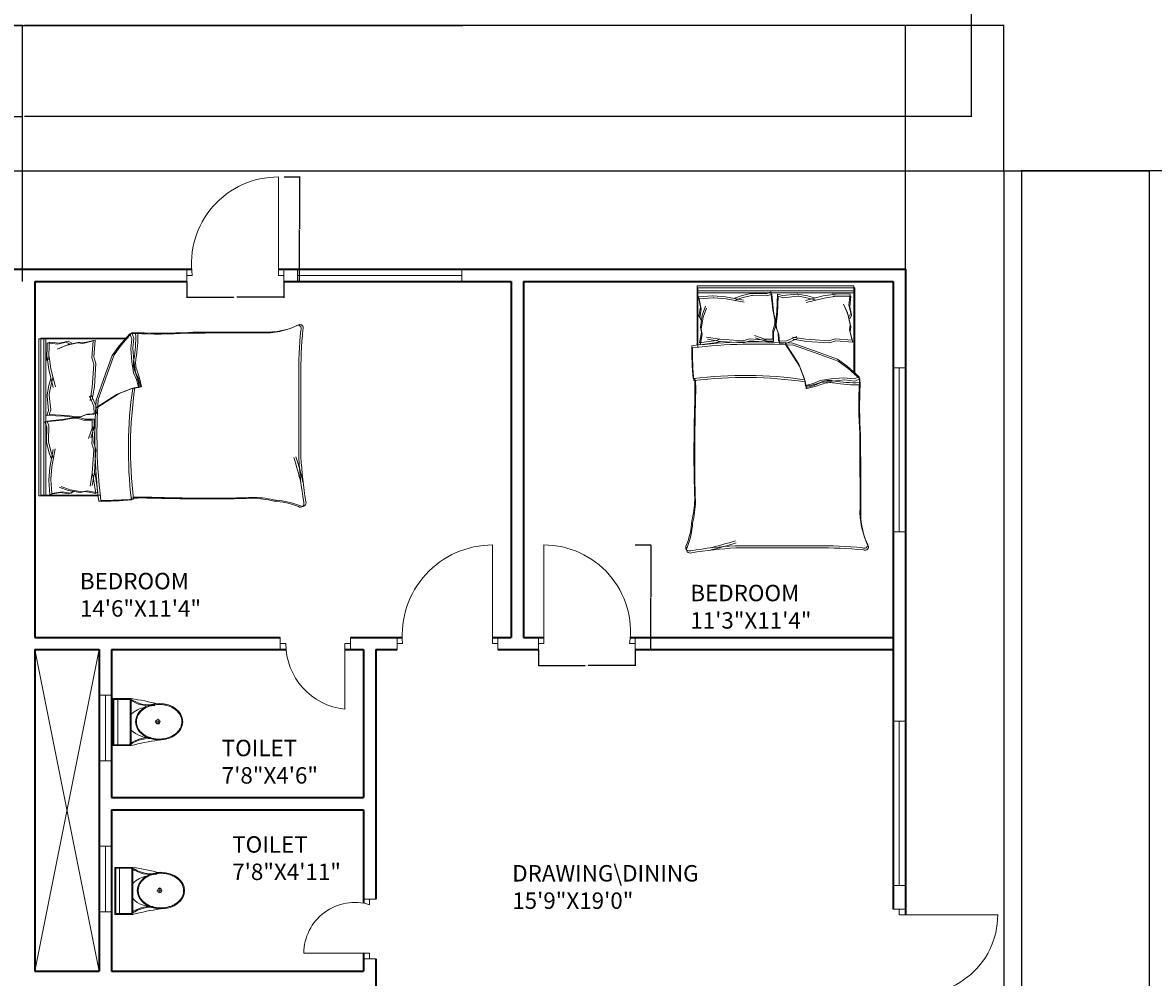
# Model space of a CAD drawing. Units: inches. Extents: x 1520 to 3401, y 1570 to 3432.
# Tile 7 of 15: x 2022 to 2435, y 2438 to 2787. Entities that reach past the tile are written whole.
import ezdxf

# ---------------------------------------------------------------- set-up
doc = ezdxf.new("R2010")
doc.units = ezdxf.units.IN
for name, color, linetype, lineweight in [('A-ANNO-DIMS', 2, 'Continuous', 18), ('A-AREA-IDEN', 7, 'Continuous', 18), ('A-DOOR', 3, 'Continuous', 18), ('A-FLOR-EDGE', 7, 'Continuous', 25), ('A-FLOR-FIXT', 9, 'Continuous', 18), ('A-FLOR-OPEN', 8, 'Continuous', 13), ('A-FURN', 8, 'Continuous', 13), ('A-GLAZ', 4, 'Continuous', 18), ('A-WALL', 7, 'Continuous', 35)]:
    doc.layers.add(name, color=color, linetype=linetype, lineweight=lineweight)
doc.styles.get("Standard").update_dxf_attribs({"font": 'arial.ttf'})
doc.dimstyles.get("Standard").update_dxf_attribs({"dimtxt": 0.18, "dimasz": 0.18, "dimexe": 0.18, "dimexo": 0.0625, "dimgap": 0.09, "dimtad": 0, "dimtih": 1, "dimtoh": 1, "dimdec": 4, "dimzin": 0, "dimdsep": 46, "dimtxsty": 'Standard', "dimcen": 0.09, "dimadec": 0, "dimazin": 0, "dimtfac": 1, "dimtdec": 4, "dimtofl": 0, "dimtmove": 0, "dimatfit": 3, "dimfxl": 1, "dimtolj": 1, "dimtzin": 0, "dimarcsym": 0})

# ---------------------------------------------------------------- blocks, each defined once
blk = doc.blocks.new('A$C31115884')
for p, q in [((258, 466), (258, 523)), ((283, 498), (223, 498)), ((0, 200), (0, 0)), ((520, 200), (0, 200)), ((10, 190), (10, 10)), ((510, 190), (10, 190)), ((510, 10), (510, 190)), ((520, 0), (520, 200)), ((510, 54), (0, 54)), ((10, 10), (510, 10)), ((0, 0), (520, 0))]:
    blk.add_line(p, q)
blk.add_circle((256, 496), 23.6)
for centre, radius, start, end in [((2778, -205), 2807, 165.4549, 171.7133), ((3237, 905), 2807, 188.2867, 194.5451), ((-295, 403), 365, 324.2091, 9.3499), ((-295, 403), 375, 324.2091, 9.3499), ((139, 406), 293, 315.8436, 2.6563), ((806, 403), 375, 179.2036, 215.7909), ((806, 403), 365, 170.6501, 215.7909), ((384, 406), 293, 190.2774, 224.1564)]:
    blk.add_arc(centre, radius, start, end)
blk.add_ellipse((256, 510), major_axis=(0, -261), ratio=0.772727)
blk.add_open_spline([(256, 259), (263, 259), (270, 260), (288, 262), (299, 265), (320, 273), (330, 278), (350, 291), (360, 299), (378, 316), (386, 326), (402, 347), (409, 358), (421, 383), (427, 395), (436, 422), (440, 436), (445, 465), (447, 480), (448, 509), (448, 524), (445, 553), (443, 568), (436, 596), (432, 610), (422, 636), (416, 649), (402, 672), (395, 683), (379, 703), (370, 712), (351, 728), (341, 735), (321, 746), (310, 751), (289, 757), (278, 759), (256, 761), (245, 761), (223, 757), (212, 754), (191, 746), (181, 741), (161, 728), (151, 720), (133, 703), (125, 693), (110, 672), (103, 660), (90, 636), (85, 623), (76, 596), (72, 582), (67, 553), (66, 538), (64, 509), (65, 494), (68, 465), (70, 450), (77, 422), (81, 408), (91, 382), (97, 370), (111, 346), (118, 335), (135, 316), (144, 307), (162, 291), (172, 284), (193, 273), (203, 269), (225, 262), (236, 260), (250, 259), (253, 259), (256, 259)], degree=3, knots=[0, 0, 0, 0, 0.110105, 0.110105, 0.285049, 0.285049, 0.459994, 0.459994, 0.634938, 0.634938, 0.809882, 0.809882, 0.984827, 0.984827, 1.159771, 1.159771, 1.334715, 1.334715, 1.50966, 1.50966, 1.684604, 1.684604, 1.859549, 1.859549, 2.034493, 2.034493, 2.209437, 2.209437, 2.384382, 2.384382, 2.559326, 2.559326, 2.73427, 2.73427, 2.909215, 2.909215, 3.084159, 3.084159, 3.259103, 3.259103, 3.434048, 3.434048, 3.608992, 3.608992, 3.783936, 3.783936, 3.958881, 3.958881, 4.133825, 4.133825, 4.30877, 4.30877, 4.483714, 4.483714, 4.658658, 4.658658, 4.833603, 4.833603, 5.008547, 5.008547, 5.183491, 5.183491, 5.358436, 5.358436, 5.53338, 5.53338, 5.708324, 5.708324, 5.883269, 5.883269, 6.058213, 6.058213, 6.233158, 6.233158, 6.283185, 6.283185, 6.283185, 6.283185])
blk = doc.blocks.new('DOOR-SWING-36-05')
for p, q in [((34.83, 2.25), (34.83, 38.25)), ((0, 4.5), (0, 4.5)), ((0, 4.5), (0, 0)), ((36.83, 4.5), (36.83, 0)), ((0, 0), (0, 2.25)), ((0, 2.25), (2, 2.25)), ((36.83, 2.25), (34.83, 2.25)), ((36.83, 0), (36.83, 2.25))]:
    blk.add_line(p, q)
blk.add_arc((34.83, 5.28), 32.97, 90, 185.2728)
blk = doc.blocks.new('DOOR-SWING-36-06')
for p, q in [((2, 2.25), (2, 38.25)), ((0, 4.5), (0, 0)), ((35.31, 4.5), (35.31, 0)), ((0, 0), (0, 2.25)), ((0, 2.25), (2, 2.25)), ((35.31, 2.25), (33.31, 2.25)), ((35.31, 0), (35.31, 2.25))]:
    blk.add_line(p, q)
blk.add_arc((2, 6.63), 31.62, 352.0372, 90)
blk = doc.blocks.new('DOOR-SWING-24-07')
for p, q in [((21.75, 21.72), (26.25, 21.72)), ((26.25, 21.72), (24, 21.72)), ((24, 21.72), (24, 19.72)), ((24, 2), (0, 2)), ((21.75, 0), (26.25, 0)), ((24, 0), (24, 2)), ((26.25, 0), (24, 0))]:
    blk.add_line(p, q)
blk.add_arc((18.54, 2), 18.54, 72.8832, 180)
blk = doc.blocks.new('DOOR-SWING-24-08')
for p, q in [((0, 26.25), (0, 21.75)), ((25.6, 21.75), (25.6, 26.25)), ((25.6, 26.25), (25.6, 24)), ((0, 21.75), (0, 24)), ((0, 24), (2, 24)), ((25.6, 24), (23.6, 24)), ((23.6, 24), (23.6, 0))]:
    blk.add_line(p, q)
blk.add_arc((26.13, 24), 24.13, 180, 263.9827)
blk = doc.blocks.new('DOOR-SWING-36-21')
for p, q in [((33.5, 2.25), (33.5, 38.25)), ((0, 4.5), (0, 0)), ((35.5, 0), (35.5, 4.5)), ((35.5, 4.5), (35.5, 2.25)), ((0, 0), (0, 2.25)), ((0, 2.25), (2, 2.25)), ((35.5, 2.25), (33.5, 2.25))]:
    blk.add_line(p, q)
blk.add_arc((33.5, 6.47), 31.78, 90, 187.6316)
blk = doc.blocks.new('DOOR-SWING-36-23')
for p, q in [((0, 32.12), (4.5, 32.12)), ((4.5, 32.12), (2.25, 32.12)), ((2.25, 32.12), (2.25, 30.12)), ((2.25, 30.12), (38.25, 30.12)), ((4.5, 0), (0, 0)), ((0, 0), (2.25, 0)), ((2.25, 0), (2.25, 2))]:
    blk.add_line(p, q)
blk.add_arc((9.27, 30.12), 28.98, 255.986, 0)
blk = doc.blocks.new('WIN-PLAN-24-01')
for p, q in [((0, 4.5), (0, 0)), ((24, 2.25), (24, 4.5)), ((24, 4.5), (24, 0)), ((0, 0), (0, 2.25)), ((0, 2.25), (24, 2.25))]:
    blk.add_line(p, q)
blk = doc.blocks.new('WIN-PLAN-60-02')
for p, q in [((4.5, 60), (0, 60)), ((0, 60), (2.25, 60)), ((2.25, 60), (2.25, 0)), ((4.5, 0), (0, 0)), ((2.25, 0), (4.5, 0))]:
    blk.add_line(p, q)
blk = doc.blocks.new('WIN-PLAN-60-03')
for p, q in [((0, 2.25), (0, 4.5)), ((0, 4.5), (0, 0)), ((60, 0), (60, 4.5)), ((60, 4.5), (60, 2.25)), ((60, 2.25), (0, 2.25))]:
    blk.add_line(p, q)
blk = doc.blocks.new('WIN-PLAN-24-07')
for p, q in [((2.25, 24), (0, 24)), ((0, 24), (4.5, 24)), ((2.25, 0), (2.25, 24)), ((4.5, 0), (0, 0)), ((0, 0), (4.5, 0)), ((4.5, 0), (2.25, 0))]:
    blk.add_line(p, q)
blk = doc.blocks.new('BED-DOUBLE')
for p, q in [((4.17, 75.93), (4.17, 97.64)), ((4.17, 97.64), (61.46, 97.64)), ((4.17, 95.8), (61.46, 95.8)), ((4.44, 75.16), (4.44, 96.87)), ((4.44, 96.87), (61.73, 96.87)), ((4.44, 95.03), (61.73, 95.03)), ((29.42, 94.7), (31.15, 95.4)), ((31.15, 95.4), (31.84, 88.98)), ((61.46, 97.64), (61.46, 65.74)), ((61.73, 96.87), (61.73, 64.97)), ((4.67, 93.64), (9.81, 94.03)), ((4.67, 93.66), (5.36, 89.85)), ((4.94, 92.9), (5.64, 89.08)), ((4.95, 92.87), (10.08, 93.27)), ((9.81, 94.03), (9.93, 94.01)), ((9.93, 94.01), (14.52, 93.66)), ((10.08, 93.27), (10.21, 93.24)), ((10.21, 93.24), (14.79, 92.9)), ((14.52, 93.66), (21.1, 92.45)), ((14.79, 92.9), (21.38, 91.68)), ((17.81, 93.14), (20.24, 94.01)), ((18.08, 92.38), (20.51, 93.24)), ((20.24, 94.01), (23.7, 94.88)), ((20.51, 93.24), (23.98, 94.11)), ((23.7, 94.88), (24.09, 94.88)), ((23.98, 94.11), (24.36, 94.11)), ((24.09, 94.88), (29.42, 94.7)), ((24.36, 94.11), (29.69, 93.94)), ((29.69, 93.94), (31.42, 94.63)), ((31.42, 94.63), (32.12, 88.22)), ((33.54, 94.65), (33.25, 88.21)), ((33.81, 93.88), (33.52, 87.44)), ((35.31, 94.07), (33.54, 94.65)), ((35.59, 93.3), (33.81, 93.88)), ((40.62, 94.57), (35.31, 94.07)), ((40.9, 93.81), (35.59, 93.3)), ((41.01, 94.6), (40.62, 94.57)), ((41.28, 93.83), (40.9, 93.81)), ((44.52, 93.95), (41.01, 94.6)), ((44.79, 93.18), (41.28, 93.83)), ((50.25, 93.96), (43.75, 92.34)), ((50.52, 93.19), (44.03, 91.57)), ((47, 93.23), (44.52, 93.95)), ((47.27, 92.47), (44.79, 93.18)), ((54.8, 94.59), (50.25, 93.96)), ((55.08, 93.82), (50.52, 93.19)), ((60.08, 94.57), (53.6, 94.69)), ((53.6, 94.69), (54.8, 94.59)), ((60.35, 93.81), (53.87, 93.92)), ((53.87, 93.92), (55.08, 93.82)), ((59.12, 87.74), (57.7, 90.95)), ((60.08, 94.57), (59.62, 90.72)), ((60.35, 93.81), (59.9, 89.96)), ((5.36, 89.85), (4.84, 86.73)), ((5.64, 89.08), (5.12, 85.96)), ((5.36, 82.57), (6.06, 86.9)), ((6.06, 86.9), (7.27, 90.2)), ((6.33, 86.14), (7.54, 89.43)), ((31.84, 88.98), (32.54, 85.17)), ((32.12, 88.22), (32.81, 84.4)), ((33.25, 88.21), (32.79, 84.36)), ((33.52, 87.44), (33.07, 83.59)), ((59.39, 86.97), (57.97, 90.18)), ((60.08, 83.46), (59.12, 87.74)), ((60.35, 82.69), (59.39, 86.97)), ((59.62, 90.72), (60.34, 87.64)), ((60.34, 87.64), (59.72, 86.39)), ((59.9, 89.96), (60.61, 86.88)), ((60.61, 86.88), (59.99, 85.62)), ((4.84, 86.73), (5.54, 85.52)), ((5.12, 85.96), (5.81, 84.75)), ((5.64, 81.8), (6.33, 86.14)), ((32.54, 83.61), (31.84, 81.36)), ((32.81, 82.84), (32.12, 80.59)), ((32.54, 85.17), (32.54, 83.61)), ((32.79, 84.36), (32.89, 82.8)), ((32.81, 84.4), (32.81, 82.84)), ((32.89, 82.8), (33.72, 80.59)), ((33.07, 83.59), (33.17, 82.03)), ((59.85, 81.53), (60.08, 83.46)), ((60.12, 80.77), (60.35, 82.69)), ((5.02, 76.85), (5.71, 80.66)), ((5.29, 76.08), (5.98, 79.9)), ((5.71, 80.66), (5.36, 82.57)), ((5.98, 79.9), (5.64, 81.8)), ((7.65, 78.9), (12.48, 78.1)), ((28.9, 78.14), (25.13, 79.45)), ((29.17, 77.37), (25.4, 78.68)), ((31.84, 81.36), (31.84, 78.14)), ((32.12, 80.59), (32.12, 77.37)), ((33.17, 82.03), (34, 79.83)), ((33.72, 80.59), (33.93, 77.39)), ((34, 79.83), (34.2, 76.62)), ((36.87, 77.57), (40.55, 79.11)), ((39.04, 78.9), (43.87, 78.1)), ((60.78, 77.77), (59.85, 81.53)), ((61.05, 77), (60.12, 80.77)), ((11.13, 77.72), (5.02, 76.85)), ((11.4, 76.95), (5.29, 76.08)), ((7.92, 78.14), (12.76, 77.34)), ((12.48, 78.1), (11.13, 77.72)), ((12.76, 77.34), (11.4, 76.95)), ((12.48, 78.1), (20.89, 77.59)), ((12.76, 77.34), (21.16, 76.82)), ((20.89, 77.59), (23.24, 78.25)), ((21.16, 76.82), (23.51, 77.49)), ((23.24, 78.25), (29.39, 77.77)), ((23.51, 77.49), (29.67, 77)), ((31.84, 78.14), (28.9, 78.14)), ((32.12, 77.37), (29.17, 77.37)), ((33.93, 77.39), (36.87, 77.57)), ((34.2, 76.62), (37.14, 76.8)), ((36.28, 76.8), (41.3, 69.01)), ((36.55, 76.03), (41.57, 68.25)), ((37.14, 76.8), (40.82, 78.34)), ((48.73, 73.28), (38.73, 76.8)), ((49, 72.52), (39, 76.03)), ((39.31, 78.14), (44.15, 77.34)), ((43.87, 78.1), (52.28, 77.59)), ((44.15, 77.34), (52.55, 76.82)), ((52.28, 77.59), (54.63, 78.25)), ((52.55, 76.82), (54.9, 77.49)), ((54.63, 78.25), (60.78, 77.77)), ((54.9, 77.49), (61.05, 77)), ((55.41, 70.87), (48.73, 73.28)), ((55.69, 70.1), (49, 72.52)), ((58.94, 68.27), (55.41, 70.87)), ((41.3, 69.01), (43.34, 63.63)), ((41.57, 68.25), (43.62, 62.87)), ((59.21, 67.51), (55.69, 70.1)), ((63.38, 64.38), (58.94, 68.27)), ((63.66, 63.61), (59.21, 67.51)), ((43.34, 63.63), (43.71, 61.22)), ((43.62, 62.87), (43.99, 60.45)), ((46.68, 61.96), (49.1, 63.08)), ((46.96, 61.2), (49.37, 62.31)), ((49.1, 63.08), (53.18, 63.63)), ((49.37, 62.31), (53.46, 62.87)), ((53.18, 63.63), (57.82, 64)), ((53.46, 62.87), (58.1, 63.24)), ((57.82, 64), (61.54, 63.63)), ((58.1, 63.24), (61.81, 62.87)), ((61.54, 63.63), (63.38, 64.38)), ((61.81, 62.87), (63.66, 63.61)), ((63.48, 62.28), (63.38, 64.38, 4.64)), ((63.75, 61.52), (63.66, 63.61, 4.64)), ((43.71, 61.22), (46.68, 61.96)), ((43.99, 60.45), (46.96, 61.2)), ((18.06, 2.64), (47.57, 2.64)), ((18.33, 1.87), (47.84, 1.87))]:
    blk.add_line(p, q)
for centre, radius, start, end in [((102.1, 73.55), 99.87, 178.7218, 185.604), ((25.61, -120.62), 197.77, 86.0865, 96.7821), ((102.37, 72.78), 99.87, 178.7218, 185.604), ((25.88, -121.38), 197.77, 86.0865, 96.7821), ((21.29, -89.76), 154.68, 81.7845, 96.9006), ((21.56, -90.53), 154.68, 81.7845, 96.9006), ((-200.58, 60.27), 203.94, 358.4762, 1.0082), ((-200.3, 59.5), 203.94, 358.4762, 1.0082), ((37.35, 95.86), 35.55, 280.6617, 289.8806), ((52.44, 55.6), 7.46, 78.6608, 113.7384), ((52.72, 54.83), 7.46, 78.6608, 113.7384), ((61.53, 105.62), 43.38, 259.8763, 272.5657), ((61.81, 104.85), 43.38, 259.8763, 272.5657), ((218.51, 54.1), 155.25, 176.9791, 183.8365), ((43.92, 61.15), 0.221, 160.2464, 271.1377), ((44.2, 60.38), 0.221, 160.2464, 271.1377), ((37.62, 95.1), 35.55, 280.6617, 289.8806), ((218.79, 53.34), 155.25, 176.9791, 183.8365), ((581.23, 36.96), 578.22, 178.22771, 181.71854), ((581.51, 36.19), 578.22, 178.22771, 181.71854), ((-5405.34, 16.33), 5469.02, 0.00217, 0.28689), ((-5405.07, 15.56), 5469.02, 0.00217, 0.28689), ((-32.25, 20.29), 35.53, 346.0648, 358.9113), ((-31.97, 19.53), 35.53, 346.0648, 358.9113), ((91.3, 15.32), 27.65, 177.4714, 206.4681), ((91.58, 14.55), 27.65, 177.4714, 206.4681), ((-25.97, 13.39), 28.25, 337.9751, 356.652), ((-25.69, 12.62), 28.25, 337.9751, 356.652), ((-20.65, 126.07), 127.63, 283.3832, 287.7053), ((1.3, 2.07), 1.31, 146.1736, 293.4781), ((1.58, 1.3), 1.31, 146.1736, 293.4781), ((25.69, -143.14), 145.97, 92.9958, 99.4091), ((25.96, -143.9), 145.97, 92.9958, 99.4091), ((-20.37, 125.3), 127.63, 283.3832, 287.7053), ((49.34, -156.85), 159.5, 84.4998, 90.6351), ((49.61, -157.62), 159.5, 84.4998, 90.6351), ((65.23, 3.08), 1.32, 242.6588, 356.02), ((65.5, 2.32), 1.32, 242.6588, 356.02)]:
    blk.add_arc(centre, radius, start, end)
blk = doc.blocks.new('*D91')
at = {"layer": 'A-ANNO-DIMS', "color": 0, "lineweight": -2, "transparency": 16777216}
for p, q in [((2245.43, 2596.43), (2251.29, 2596.43)), ((2251.11, 2596.25), (2251.11, 2577.49)), ((2251.11, 2558.36), (2251.11, 2577.12)), ((2245.43, 2558.18), (2251.29, 2558.18))]:
    blk.add_line(p, q, dxfattribs=at)
at = {"layer": 'A-ANNO-DIMS', "color": 0, "transparency": 16777216}
for points in [[(2251.08, 2596.25), (2251.14, 2596.25), (2251.11, 2596.43)], [(2251.08, 2558.36), (2251.14, 2558.36), (2251.11, 2558.18)]]:
    blk.add_solid(points, dxfattribs=at)
at = {"layer": 'Defpoints', "color": 0, "transparency": 16777216}
for p in [(2245.37, 2596.43), (2251.11, 2596.43), (2245.37, 2558.18)]:
    blk.add_point(p, dxfattribs=at)
at = {"layer": 'A-ANNO-DIMS', "color": 0, "transparency": 16777216, "insert": (2251.11, 2577.3), "char_height": 0.18, "attachment_point": 5}
blk.add_mtext('\\A1;D06 38 TYP.', dxfattribs=at)
blk = doc.blocks.new('*D92')
at = {"layer": 'A-ANNO-DIMS', "color": 0, "lineweight": -2, "transparency": 16777216}
for p, q in [((2210.05, 2558.12), (2210.05, 2552.26)), ((2245.37, 2558.12), (2245.37, 2552.26)), ((2210.23, 2552.44), (2227.18, 2552.44)), ((2245.19, 2552.44), (2228.24, 2552.44))]:
    blk.add_line(p, q, dxfattribs=at)
at = {"layer": 'A-ANNO-DIMS', "color": 0, "transparency": 16777216}
for points in [[(2210.23, 2552.47), (2210.23, 2552.41), (2210.05, 2552.44)], [(2245.19, 2552.47), (2245.19, 2552.41), (2245.37, 2552.44)]]:
    blk.add_solid(points, dxfattribs=at)
at = {"layer": 'Defpoints', "color": 0, "transparency": 16777216}
for p in [(2210.05, 2558.18), (2245.37, 2558.18), (2245.37, 2552.44)]:
    blk.add_point(p, dxfattribs=at)
at = {"layer": 'A-ANNO-DIMS', "color": 0, "transparency": 16777216, "insert": (2227.71, 2552.44), "char_height": 0.18, "attachment_point": 5}
blk.add_mtext('\\A1;35 TYP.', dxfattribs=at)
blk = doc.blocks.new('*D121')
at = {"layer": 'A-ANNO-DIMS', "color": 0, "lineweight": -2, "transparency": 16777216}
for p, q in [((2117.14, 2730.93), (2122.99, 2730.93)), ((2122.81, 2730.75), (2122.81, 2711.99)), ((2122.81, 2692.86), (2122.81, 2711.62)), ((2117.14, 2692.68), (2122.99, 2692.68))]:
    blk.add_line(p, q, dxfattribs=at)
at = {"layer": 'A-ANNO-DIMS', "color": 0, "transparency": 16777216}
for points in [[(2122.78, 2730.75), (2122.84, 2730.75), (2122.81, 2730.93)], [(2122.78, 2692.86), (2122.84, 2692.86), (2122.81, 2692.68)]]:
    blk.add_solid(points, dxfattribs=at)
at = {"layer": 'Defpoints', "color": 0, "transparency": 16777216}
for p in [(2117.08, 2730.93), (2122.81, 2730.93), (2117.08, 2692.68)]:
    blk.add_point(p, dxfattribs=at)
at = {"layer": 'A-ANNO-DIMS', "color": 0, "transparency": 16777216, "insert": (2122.81, 2711.8), "char_height": 0.18, "attachment_point": 5}
blk.add_mtext('\\A1;D21 38 TYP.', dxfattribs=at)
blk = doc.blocks.new('*D122')
at = {"layer": 'A-ANNO-DIMS', "color": 0, "lineweight": -2, "transparency": 16777216}
for p, q in [((2081.58, 2692.62), (2081.58, 2686.76)), ((2117.08, 2692.62), (2117.08, 2686.76)), ((2081.76, 2686.94), (2098.8, 2686.94)), ((2116.9, 2686.94), (2099.85, 2686.94))]:
    blk.add_line(p, q, dxfattribs=at)
at = {"layer": 'A-ANNO-DIMS', "color": 0, "transparency": 16777216}
for points in [[(2081.76, 2686.97), (2081.76, 2686.91), (2081.58, 2686.94)], [(2116.9, 2686.97), (2116.9, 2686.91), (2117.08, 2686.94)]]:
    blk.add_solid(points, dxfattribs=at)
at = {"layer": 'Defpoints', "color": 0, "transparency": 16777216}
for p in [(2081.58, 2692.68), (2117.08, 2692.68), (2117.08, 2686.94)]:
    blk.add_point(p, dxfattribs=at)
at = {"layer": 'A-ANNO-DIMS', "color": 0, "transparency": 16777216, "insert": (2099.33, 2686.94), "char_height": 0.18, "attachment_point": 5}
blk.add_mtext('\\A1;35 TYP.', dxfattribs=at)
blk = doc.blocks.new('*D181')
at = {"layer": 'A-ANNO-DIMS', "color": 0, "lineweight": -2, "transparency": 16777216}
for p, q in [((1663.61, 2733.24), (1663.61, 2786.46)), ((1663.79, 2786.28), (2021.47, 2786.28)), ((2379.93, 2786.28), (2022.26, 2786.28)), ((2380.11, 2733.24), (2380.11, 2786.46))]:
    blk.add_line(p, q, dxfattribs=at)
at = {"layer": 'A-ANNO-DIMS', "color": 0, "transparency": 16777216}
for points in [[(1663.79, 2786.31), (1663.79, 2786.25), (1663.61, 2786.28)], [(2379.93, 2786.31), (2379.93, 2786.25), (2380.11, 2786.28)]]:
    blk.add_solid(points, dxfattribs=at)
at = {"layer": 'Defpoints', "color": 0, "transparency": 16777216}
for p in [(2380.11, 2786.28), (1663.61, 2733.18), (2380.11, 2733.18)]:
    blk.add_point(p, dxfattribs=at)
at = {"layer": 'A-ANNO-DIMS', "color": 0, "transparency": 16777216, "insert": (2021.86, 2786.28), "char_height": 0.18, "attachment_point": 5}
blk.add_mtext('\\A1;716.5', dxfattribs=at)
blk = doc.blocks.new('*D182')
at = {"layer": 'A-ANNO-DIMS', "color": 0, "lineweight": -2, "transparency": 16777216}
for p, q in [((2380.18, 2733.18), (2433.39, 2733.18)), ((2433.21, 2733), (2433.21, 2244.61)), ((2433.21, 1755.86), (2433.21, 2244.25)), ((2344.18, 1755.68), (2433.39, 1755.68))]:
    blk.add_line(p, q, dxfattribs=at)
at = {"layer": 'A-ANNO-DIMS', "color": 0, "transparency": 16777216}
for points in [[(2433.18, 2733), (2433.24, 2733), (2433.21, 2733.18)], [(2433.18, 1755.86), (2433.24, 1755.86), (2433.21, 1755.68)]]:
    blk.add_solid(points, dxfattribs=at)
at = {"layer": 'Defpoints', "color": 0, "transparency": 16777216}
for p in [(2380.11, 2733.18), (2344.11, 1755.68), (2433.21, 1755.68)]:
    blk.add_point(p, dxfattribs=at)
at = {"layer": 'A-ANNO-DIMS', "color": 0, "transparency": 16777216, "insert": (2433.21, 2244.43), "char_height": 0.18, "attachment_point": 5}
blk.add_mtext('\\A1;977.5', dxfattribs=at)
blk = doc.blocks.new('*D183')
at = {"layer": 'A-ANNO-DIMS', "color": 0, "lineweight": -2, "transparency": 16777216}
for p, q in [((1699.61, 2697.24), (1699.61, 2786.46)), ((1699.79, 2786.28), (1860.32, 2786.28)), ((2021.43, 2786.28), (1860.9, 2786.28)), ((2021.61, 2692.74), (2021.61, 2786.46))]:
    blk.add_line(p, q, dxfattribs=at)
at = {"layer": 'A-ANNO-DIMS', "color": 0, "transparency": 16777216}
for points in [[(1699.79, 2786.31), (1699.79, 2786.25), (1699.61, 2786.28)], [(2021.43, 2786.31), (2021.43, 2786.25), (2021.61, 2786.28)]]:
    blk.add_solid(points, dxfattribs=at)
at = {"layer": 'Defpoints', "color": 0, "transparency": 16777216}
for p in [(2021.61, 2786.28), (1699.61, 2697.18), (2021.61, 2692.68)]:
    blk.add_point(p, dxfattribs=at)
at = {"layer": 'A-ANNO-DIMS', "color": 0, "transparency": 16777216, "insert": (1860.61, 2786.28), "char_height": 0.18, "attachment_point": 5}
blk.add_mtext('\\A1;322', dxfattribs=at)
blk = doc.blocks.new('*D184')
at = {"layer": 'A-ANNO-DIMS', "color": 0, "lineweight": -2, "transparency": 16777216}
for p, q in [((2021.61, 2692.74), (2021.61, 2786.46)), ((2021.79, 2786.28), (2182.47, 2786.28)), ((2343.93, 2786.28), (2183.26, 2786.28)), ((2344.11, 2697.24), (2344.11, 2786.46))]:
    blk.add_line(p, q, dxfattribs=at)
at = {"layer": 'A-ANNO-DIMS', "color": 0, "transparency": 16777216}
for points in [[(2021.79, 2786.31), (2021.79, 2786.25), (2021.61, 2786.28)], [(2343.93, 2786.31), (2343.93, 2786.25), (2344.11, 2786.28)]]:
    blk.add_solid(points, dxfattribs=at)
at = {"layer": 'Defpoints', "color": 0, "transparency": 16777216}
for p in [(2344.11, 2786.28), (2344.11, 2697.18), (2021.61, 2692.68)]:
    blk.add_point(p, dxfattribs=at)
at = {"layer": 'A-ANNO-DIMS', "color": 0, "transparency": 16777216, "insert": (2182.86, 2786.28), "char_height": 0.18, "attachment_point": 5}
blk.add_mtext('\\A1;322.5', dxfattribs=at)
blk = doc.blocks.new('*D192')
at = {"layer": 'A-ANNO-DIMS', "color": 0, "lineweight": -2, "transparency": 16777216}
for p, q in [((2467.84, 2733.18), (2386.32, 2733.18)), ((2386.5, 2733), (2386.5, 2244.61)), ((2386.5, 1755.86), (2386.5, 2244.25)), ((2503.84, 1755.68), (2386.32, 1755.68))]:
    blk.add_line(p, q, dxfattribs=at)
at = {"layer": 'A-ANNO-DIMS', "color": 0, "transparency": 16777216}
for points in [[(2386.47, 2733), (2386.53, 2733), (2386.5, 2733.18)], [(2386.47, 1755.86), (2386.53, 1755.86), (2386.5, 1755.68)]]:
    blk.add_solid(points, dxfattribs=at)
at = {"layer": 'Defpoints', "color": 0, "transparency": 16777216}
for p in [(2467.9, 2733.18), (2386.5, 1755.68), (2503.9, 1755.68)]:
    blk.add_point(p, dxfattribs=at)
at = {"layer": 'A-ANNO-DIMS', "color": 0, "transparency": 16777216, "insert": (2386.5, 2244.43), "char_height": 0.18, "attachment_point": 5}
blk.add_mtext('\\A1;977.5', dxfattribs=at)
blk = doc.blocks.new('*D209')
at = {"layer": 'A-ANNO-DIMS', "color": 0, "lineweight": -2, "transparency": 16777216}
for p, q in [((1675.61, 3007.57), (1675.61, 2752.86)), ((2368.11, 3007.57), (2368.11, 2752.86)), ((1675.79, 2753.04), (2021.47, 2753.04)), ((2367.93, 2753.04), (2022.26, 2753.04))]:
    blk.add_line(p, q, dxfattribs=at)
at = {"layer": 'A-ANNO-DIMS', "color": 0, "transparency": 16777216}
for points in [[(1675.79, 2753.07), (1675.79, 2753.01), (1675.61, 2753.04)], [(2367.93, 2753.07), (2367.93, 2753.01), (2368.11, 2753.04)]]:
    blk.add_solid(points, dxfattribs=at)
at = {"layer": 'Defpoints', "color": 0, "transparency": 16777216}
for p in [(1675.61, 3007.63), (2368.11, 3007.63), (2368.11, 2753.04)]:
    blk.add_point(p, dxfattribs=at)
at = {"layer": 'A-ANNO-DIMS', "color": 0, "transparency": 16777216, "insert": (2021.86, 2753.04), "char_height": 0.18, "attachment_point": 5}
blk.add_mtext('\\A1;692.5', dxfattribs=at)

msp = doc.modelspace()

# ---------------------------------------------------------------- linework, layer by layer
at = {"layer": 'A-FLOR-EDGE'}
for p, q in [((1663.6128, 2733.1786), (2380.1128, 2733.1786)), ((2380.1128, 2733.1786), (2380.1128, 1791.6786))]:
    msp.add_line(p, q, dxfattribs=at)
at = {"layer": 'A-FLOR-OPEN'}
for p, q in [((2049.6128, 2558.1786), (2026.1128, 2440.6786)), ((2026.1128, 2558.1786), (2049.6128, 2440.6786))]:
    msp.add_line(p, q, dxfattribs=at)
at = {"layer": 'A-WALL'}
for p, q in [((1807.4069, 2697.1786), (2083.3571, 2697.1786)), ((2115.0755, 2697.1786), (2344.1128, 2697.1786)), ((2344.1128, 2697.1786), (2344.1128, 2461.3065)), ((2026.1128, 2692.6786), (2026.1128, 2562.6786)), ((2026.1128, 2692.6786), (2081.5774, 2692.6786)), ((2117.0755, 2692.6786), (2200.1128, 2692.6786)), ((2200.1128, 2692.6786), (2200.1128, 2562.6786)), ((2204.6128, 2692.6786), (2204.6128, 2562.6786)), ((2204.6128, 2692.6786), (2339.6128, 2692.6786)), ((2339.6128, 2692.6786), (2339.6128, 2463.3065)), ((2026.1128, 2562.6786), (2115.7596, 2562.6786)), ((2141.3627, 2562.6786), (2160.3046, 2562.6786)), ((2193.2655, 2562.6786), (2200.1128, 2562.6786)), ((2204.6128, 2562.6786), (2212.0528, 2562.6786)), ((2243.6006, 2562.6786), (2339.6128, 2562.6786)), ((2026.1128, 2558.1786), (2026.1128, 2440.6786)), ((2026.1128, 2558.1786), (2049.6128, 2558.1786)), ((2049.6128, 2558.1786), (2049.6128, 2440.6786)), ((2054.1128, 2558.1786), (2054.1128, 2504.1786)), ((2054.1128, 2558.1786), (2117.8647, 2558.1786)), ((2139.3627, 2558.1786), (2146.1128, 2558.1786)), ((2146.1128, 2558.1786), (2146.1128, 2504.1786)), ((2150.6128, 2558.1786), (2150.6128, 2466.9777)), ((2150.6128, 2558.1786), (2158.4349, 2558.1786)), ((2195.2655, 2558.1786), (2210.0528, 2558.1786)), ((2245.3676, 2558.1786), (2339.6128, 2558.1786)), ((2054.1128, 2504.1786), (2146.1128, 2504.1786)), ((2054.1128, 2499.6786), (2146.1128, 2499.6786)), ((2054.1128, 2499.6786), (2054.1128, 2440.6786)), ((2146.1128, 2499.6786), (2146.1128, 2465.5195)), ((2146.1128, 2447.2565), (2146.1128, 2440.6786)), ((2150.6128, 2445.2565), (2150.6128, 2424.6989)), ((2026.1128, 2440.6786), (2049.6128, 2440.6786)), ((2054.1128, 2440.6786), (2146.1128, 2440.6786))]:
    msp.add_line(p, q, dxfattribs=at)

# ---------------------------------------------------------------- block references
at = {"layer": 'A-DOOR'}
for name, p in [('DOOR-SWING-36-21', (2081.577, 2692.679)), ('DOOR-SWING-36-05', (2158.435, 2558.179)), ('DOOR-SWING-36-06', (2210.053, 2558.179)), ('DOOR-SWING-24-08', (2115.76, 2536.429)), ('DOOR-SWING-24-07', (2124.363, 2445.256)), ('DOOR-SWING-36-23', (2339.613, 2431.187))]:
    msp.add_blockref(name, p, dxfattribs=at)
at = {"layer": 'A-FLOR-FIXT', "xscale": 0.0330640103915726, "yscale": 0.0330640103915726, "zscale": 0.0330640103915726, "rotation": 270}
for p in [(2054.6303, 2540.3006), (2055.2775, 2478.6225)]:
    msp.add_blockref('A$C31115884', p, dxfattribs=at)
at = {"layer": 'A-FURN'}
msp.add_blockref('BED-DOUBLE', (2263.8598, 2593.4746), dxfattribs=at)
at = {"layer": 'A-FURN', "rotation": 90.00000000000003}
msp.add_blockref('BED-DOUBLE', (2125.1645, 2610.2383), dxfattribs=at)
at = {"layer": 'A-GLAZ'}
for name, p in [('WIN-PLAN-60-03', (2122.086, 2692.679)), ('WIN-PLAN-24-07', (2049.613, 2517.567))]:
    msp.add_blockref(name, p, dxfattribs=at)
at = {"layer": 'A-GLAZ', "extrusion": (0, 0, -1), "zscale": -1}
for name, p, rotation in [('WIN-PLAN-60-02', (-2339.613, 2661.184), 180), ('WIN-PLAN-60-03', (-2339.6132, 2472.0145), 90)]:
    msp.add_blockref(name, p, dxfattribs=dict(at, rotation=rotation))
at = {"layer": 'A-GLAZ', "rotation": 270}
msp.add_blockref('WIN-PLAN-24-01', (2049.6132, 2486.4027), dxfattribs=at)

# ---------------------------------------------------------------- texts
at = {"layer": 'A-AREA-IDEN', "char_height": 6, "attachment_point": 1}
for s, width, insert in [('BEDROOM\\P14\'6"X11\'4"', 108.040202, (2042.541, 2586.238)), ('BEDROOM\\P11\'3"X11\'4"', 114.584941, (2265.5279, 2581.8709)), ('TOILET\\P7\'8"X4\'6"', 109.697721, (2094.3498, 2525.2454)), ('TOILET\\P7\'8"X4\'11"', 80.378615, (2098.1859, 2490.0053)), ('DRAWING\\\\DINING\\P15\'9"X19\'0"', 113.529906, (2200.479, 2479.4626))]:
    msp.add_mtext_dynamic_manual_height_columns(s, width=width, gutter_width=12.5, heights=[0], dxfattribs=dict(at, insert=insert))

# ---------------------------------------------------------------- dimensions: what is measured, and where the dimension line sits
at = {"layer": 'A-ANNO-DIMS'}
for base, p1, p2, override, picture, middle in [((2368.1128, 2753.0384), (1675.6128, 3007.633), (2368.1128, 3007.633), {"dimdec": 1, "dimlfac": 1, "dimrnd": 0, "dimzin": 0, "dimdsep": 46, "dimlunit": 2}, '*D209', (2021.8628, 2753.0384)), ((2380.1128, 2786.2786), (1663.6128, 2733.1786), (2380.1128, 2733.1786), {"dimdec": 1, "dimlfac": 1, "dimrnd": 0, "dimzin": 0, "dimdsep": 46, "dimlunit": 2}, '*D181', (2021.8628, 2786.2786)), ((2021.6128, 2786.2786), (1699.6128, 2697.1786), (2021.6128, 2692.6786), {"dimdec": 0, "dimlfac": 1, "dimrnd": 0, "dimzin": 0, "dimdsep": 46, "dimlunit": 2}, '*D183', (1860.6128, 2786.2786)), ((2344.1128, 2786.2786), (2021.6128, 2692.6786), (2344.1128, 2697.1786), {"dimdec": 1, "dimlfac": 1, "dimrnd": 0, "dimzin": 0, "dimdsep": 46, "dimlunit": 2}, '*D184', (2182.8628, 2786.2786))]:
    dim = msp.add_linear_dim(base=base, p1=p1, p2=p2, dimstyle='Standard', override=override, dxfattribs=at)
    dim.commit()
    dim.dimension.update_dxf_attribs({"geometry": picture, "text_midpoint": middle})
for base, p1, p2, text, picture, middle in [((2122.813, 2730.9286), (2117.0755, 2692.6786), (2117.0755, 2730.9286), 'D21 <> TYP.', '*D121', (2122.813, 2711.8036)), ((2251.1051, 2596.4286), (2245.3676, 2558.1786), (2245.3676, 2596.4286), 'D06 <> TYP.', '*D91', (2251.1051, 2577.3036))]:
    dim = msp.add_linear_dim(base=base, p1=p1, p2=p2, angle=90, text=text, dimstyle='Standard', override={"dimdec": 0, "dimlfac": 1, "dimrnd": 0, "dimzin": 0, "dimdsep": 46, "dimlunit": 2}, dxfattribs=at)
    dim.commit()
    dim.dimension.update_dxf_attribs({"geometry": picture, "text_midpoint": middle})
for base, p1, p2, picture, middle in [((2433.2128, 1755.6786), (2380.1128, 2733.1786), (2344.1128, 1755.6786), '*D182', (2433.2128, 2244.4286)), ((2386.4982, 1755.6786), (2467.8987, 2733.1786), (2503.8987, 1755.6786), '*D192', (2386.4982, 2244.4286))]:
    dim = msp.add_linear_dim(base=base, p1=p1, p2=p2, angle=90, dimstyle='Standard', override={"dimdec": 1, "dimlfac": 1, "dimrnd": 0, "dimzin": 0, "dimdsep": 46, "dimlunit": 2}, dxfattribs=at)
    dim.commit()
    dim.dimension.update_dxf_attribs({"geometry": picture, "text_midpoint": middle})
for base, p1, p2, picture, middle in [((2117.0755, 2686.9411), (2081.5774, 2692.6786), (2117.0755, 2692.6786), '*D122', (2099.3265, 2686.9411)), ((2245.3676, 2552.4411), (2210.0528, 2558.1786), (2245.3676, 2558.1786), '*D92', (2227.7102, 2552.4411))]:
    dim = msp.add_linear_dim(base=base, p1=p1, p2=p2, text='<> TYP.', dimstyle='Standard', override={"dimdec": 0, "dimlfac": 1, "dimrnd": 0, "dimzin": 0, "dimdsep": 46, "dimlunit": 2}, dxfattribs=at)
    dim.commit()
    dim.dimension.update_dxf_attribs({"geometry": picture, "text_midpoint": middle})

doc.saveas('drawing.dxf')
